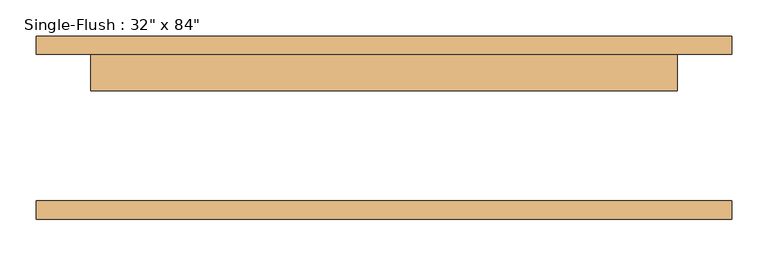
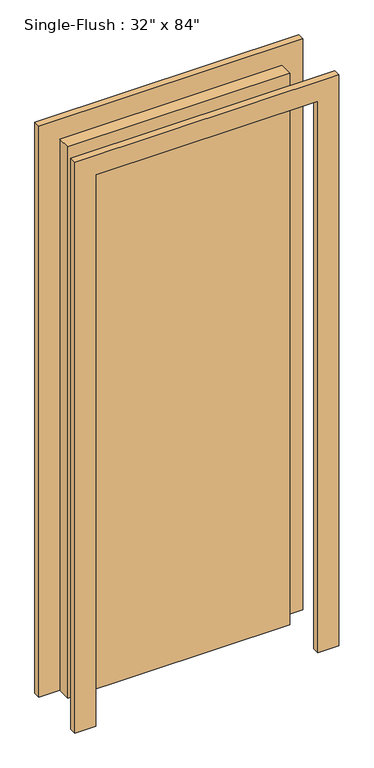
"""IFC4 building model written with IfcOpenShell, lengths in millimetres: door geometry."""

from ifc_helpers import new_model, si_unit, frame, origin, origin_with_axes, place, context, project, spatial, polyline, outline, extrude, source, transform, mapped, element, save


def door_64d5ae29(model_context):
    return source(origin(), model_context, "Body", "SweptSolid", [
        extrude(outline(polyline([(2209.8, -482.6), (0.0, -482.6), (0.0, -406.4), (2133.6, -406.4), (2133.6, 406.4), (0.0, 406.4), (0.0, 482.6), (2209.8, 482.6), (2209.8, -482.6)])), frame((0.0, 101.6, 0.0), z_axis=(0.0, 1.0, 0.0), x_axis=(0.0, 0.0, 1.0)), (0.0, 0.0, 1.0), 25.4),
        extrude(outline(polyline([(2209.8, 482.6), (2209.8, -482.6), (0.0, -482.6), (0.0, -406.4), (2133.6, -406.4), (2133.6, 406.4), (0.0, 406.4), (0.0, 482.6), (2209.8, 482.6)])), frame((0.0, -127.0, 0.0), z_axis=(0.0, 1.0, 0.0), x_axis=(0.0, 0.0, 1.0)), (0.0, 0.0, 1.0), 25.4),
        extrude(outline(polyline([(406.4, 50.8), (-406.4, 50.8), (-406.4, 101.6), (406.4, 101.6), (406.4, 50.8)])), origin_with_axes(), (0.0, 0.0, 1.0), 2133.6),
    ])


if __name__ == "__main__":
    model = new_model("IFC4")
    model_context = context("Model", 3, world=origin())
    ifc_project = project(units=[si_unit("LENGTHUNIT", "METRE", prefix="MILLI")], contexts=[model_context])
    site = spatial("IfcSite", under=ifc_project)
    building = spatial("IfcBuilding", under=site)
    placement = place(None, origin())
    door_shape = door_64d5ae29(model_context)
    element("IfcDoor", 1, ObjectType="Single-Flush : 32\" x 84\"", at=placement, inside=building, context=model_context, shape_type="MappedRepresentation", body=[
        mapped(door_shape, transform((0.0, 0.0, 0.0), x_axis=(1.0, 0.0, 0.0), y_axis=(0.0, 1.0, 0.0), z_axis=(0.0, 0.0, 1.0))),
    ])
    save(model, "model.ifc")

# Revit data of these elements
# Type "Single-Flush : 32\" x 84\""
#   Type Mark = "3"
#   Construction Type Id = "MDOOR"
#   Assembly Code = "C1020"
#   Analytic Construction = "Metal"
#   Thickness = 0' - 2"
#   Heat Transfer Coefficient (U) = 0.651978 BTU/(h·ft²·°F)
#   Height = 7' - 0"
#   Trim Projection Ext = 0' - 1"
#   Trim Projection Int = 0' - 1"
#   Trim Width = 0' - 3"
#   Width = 2' - 8"
#   Define Thermal Properties by = 1
#   Door Material = Door - Panel
#   Frame Material = Door - Frame
#   Visual Light Transmittance = 0
#   Solar Heat Gain Coefficient = 0
#   Function = (empty or 0)
#   Wall Closure = (empty or 0)
# Element 1 (IfcDoor, "Single-Flush : 32\" x 84\"")
#   Materials on its faces: "Door - Frame", "Door - Panel"
# Materials
#   "Door - Panel": class "Wood", colour RGB 210 159 95, transparency 0
#   "Door - Frame": colour RGB 118 70 51, transparency 0
